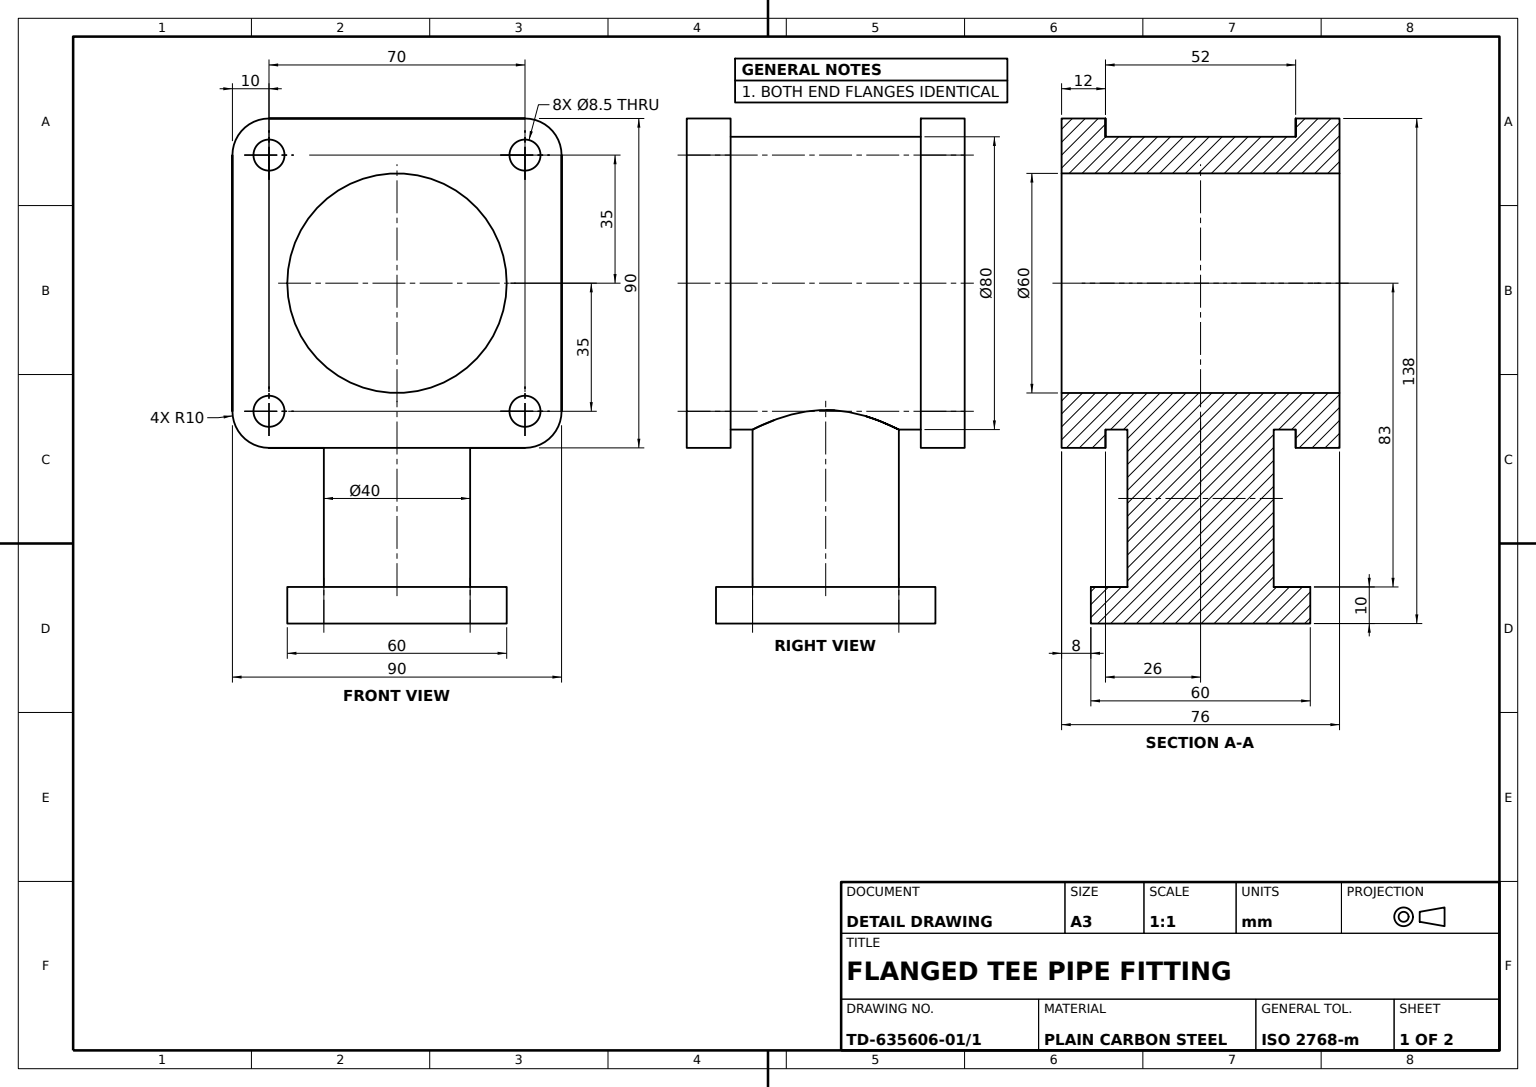
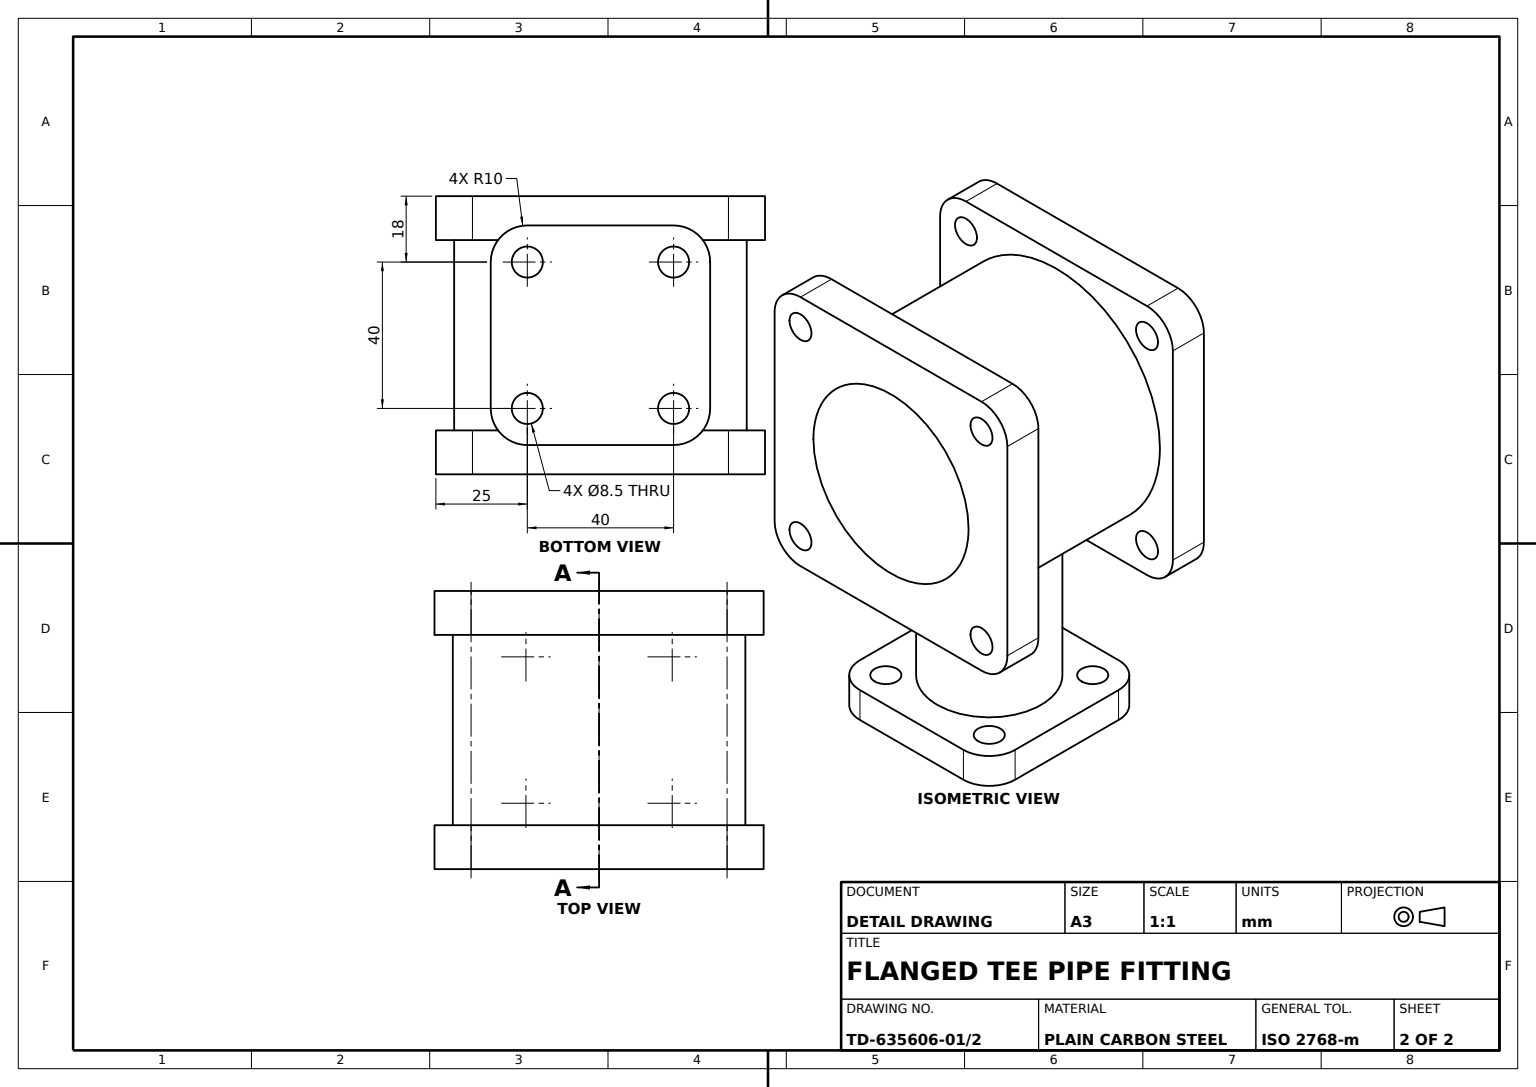
SolidWorks part; units mm, degrees
material "Plain Carbon Steel"
ref_plane "Front Plane" through (0, 0, 0) normal (0, 0, 1) x (1, 0, 0)
ref_plane "Top Plane" through (0, 0, 0) normal (0, 1, 0) x (1, 0, 0)
ref_plane "Right Plane" through (0, 0, 0) normal (1, 0, 0) x (0, 0, -1)
sketch "Body Tube Sketch" plane through (0, 0, 0) normal (0, 0, 1) x (1, 0, 0)
  circle A0 centre (0, 0) radius 30
  circle A1 centre (0, 0) radius 40
  dimension "D1" = 60
  dimension "D2" = 80
extrude "Body Tube Ø80" add sketch "Body Tube Sketch" along normal blind 52
ref_plane "Plane2" through (0, 0, 0) normal (0, 0, 1) x (1, 0, 0)
sketch "Inlet Flange Sketch" plane through (0, 0, 0) normal (0, 0, 1) x (1, 0, 0)
  line L1 (45, 45) -> (-45, 45)
  line L2 (45, 45) -> (45, -45)
  line L3 (45, -45) -> (-45, -45)
  line L4 (-45, 45) -> (-45, -45)
  line L5 (45, 45) -> (-45, -45) construction
  line L6 (45, -45) -> (-45, 45) construction
  point P0 (0, 0)
  dimension "D1" = 90
  dimension "D2" = 90
extrude "Inlet Flange 90x90" add sketch "Inlet Flange Sketch" against normal blind 12
ref_plane "Plane5" through (0, 0, 52) normal (0, 0, 1) x (1, 0, 0)
sketch "Outlet Flange Sketch" plane through (0, 0, 52) normal (0, 0, 1) x (1, 0, 0)
  line L1 (-45, 45) -> (45, 45)
  line L2 (-45, 45) -> (-45, -45)
  line L3 (-45, -45) -> (45, -45)
  line L4 (45, 45) -> (45, -45)
  line L5 (-45, 45) -> (45, -45) construction
  line L6 (-45, -45) -> (45, 45) construction
  point P0 (0, 0)
  dimension "D1" = 90
  dimension "D2" = 90
extrude "Outlet Flange 90x90" add sketch "Outlet Flange Sketch" along normal blind 12
sketch "Flange Bore Sketch" plane through (0, 0, 64) normal (0, 0, 1) x (1, 0, 0)
  circle A0 centre (0, 0) radius 30
  dimension "D1" = 60
extrude "Flange Bore Ø60" cut sketch "Flange Bore Sketch" against normal through all
fillet "Outlet Flange Corner Fillets R10" radius 10 4 edges at (-45, -45, 58) (45, -45, 58) (45, 45, 58) (-45, 45, 58)
fillet "Inlet Flange Corner Fillets R10" radius 10 4 edges at (45, -45, -6) (-45, -45, -6) (-45, 45, -6) (45, 45, -6)
sketch "Inlet Flange Holes Sketch" plane through (0, 0, -12) normal (0, 0, -1) x (-1, 0, 0)
  circle A0 centre (-35, 35) radius 4.25
  circle A1 centre (35, 35) radius 4.25
  circle A2 centre (35, -35) radius 4.25
  circle A3 centre (-35, -35) radius 4.25
  dimension "D1" = 8.5
  dimension "D2" = 8.5
  dimension "D3" = 8.5
  dimension "D4" = 8.5
extrude "Inlet Flange Holes 4xØ8.5" cut sketch "Inlet Flange Holes Sketch" against normal blind 12
sketch "Outlet Flange Holes Sketch" plane through (0, 0, 64) normal (0, 0, 1) x (1, 0, 0)
  circle A0 centre (-35, 35) radius 4.25
  circle A1 centre (35, 35) radius 4.25
  circle A2 centre (35, -35) radius 4.25
  circle A3 centre (-35, -35) radius 4.25
  dimension "D1" = 8.5
  dimension "D2" = 8.5
  dimension "D3" = 8.5
  dimension "D4" = 8.5
extrude "Outlet Flange Holes 4xØ8.5" cut sketch "Outlet Flange Holes Sketch" against normal blind 12
ref_plane "Plane6" through (0, -83, 0) normal (0, 1, 0) x (1, 0, 0)
sketch "Branch Pipe Sketch" plane through (0, -83, 0) normal (0, 1, 0) x (1, 0, 0)
  circle A0 centre (0, -26) radius 20
  dimension "D1" = 40
  dimension "D2" = 26
extrude "Branch Pipe Ø40" add sketch "Branch Pipe Sketch" along normal blind 50
sketch "Mounting Foot Sketch" plane through (0, -83, 0) normal (0, 1, 0) x (1, 0, 0)
  line L1 (-30, -56) -> (30, -56)
  line L2 (-30, -56) -> (-30, 4)
  line L3 (-30, 4) -> (30, 4)
  line L4 (30, -56) -> (30, 4)
  line L5 (-30, -56) -> (30, 4) construction
  line L6 (-30, 4) -> (30, -56) construction
  point P0 (0, -26)
  dimension "D1" = 60
  dimension "D2" = 60
extrude "Mounting Foot 60x60" add sketch "Mounting Foot Sketch" against normal blind 10
fillet "Mounting Foot Corner Fillets R10" radius 10 4 edges at (-30, -88, 56) (30, -88, 56) (30, -88, -4) (-30, -88, -4)
sketch "Mounting Foot Holes Sketch" plane through (0, -93, 0) normal (0, -1, 0) x (1, 0, 0)
  circle A0 centre (-20, 46) radius 4.25
  circle A1 centre (20, 46) radius 4.25
  circle A2 centre (20, 6) radius 4.25
  circle A3 centre (-20, 6) radius 4.25
  dimension "D1" = 8.5
  dimension "D2" = 8.5
  dimension "D3" = 8.5
  dimension "D4" = 8.5
extrude "Mounting Foot Holes 4xØ8.5" cut sketch "Mounting Foot Holes Sketch" against normal blind 10
